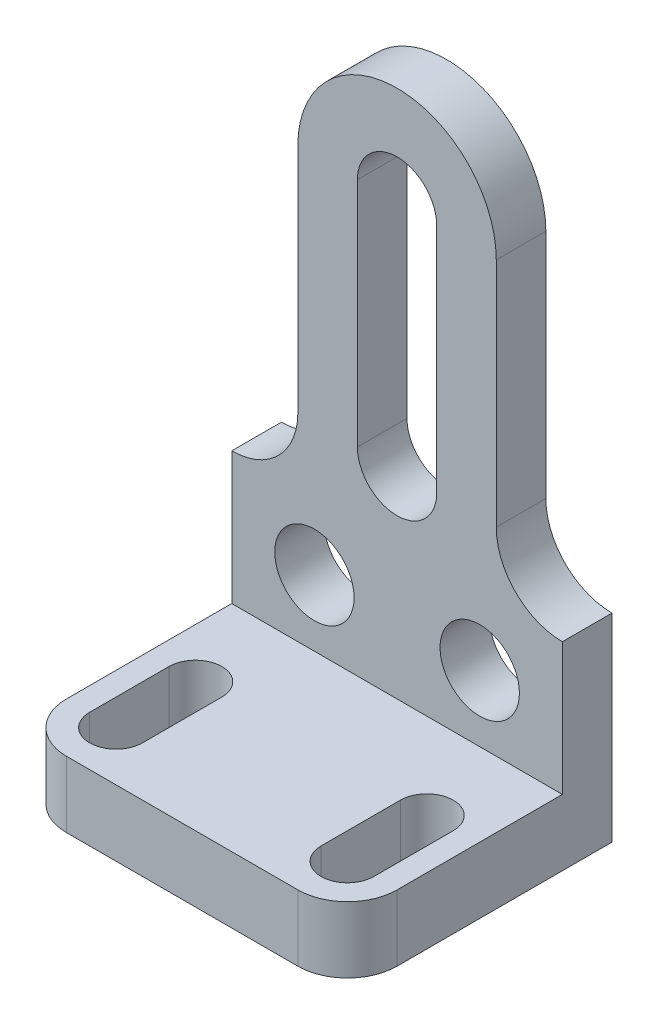
ISO-10303-21;
HEADER;
FILE_DESCRIPTION(('STEP AP214'),'2;1');
FILE_NAME('part.step','',(''),(''),'','','');
FILE_SCHEMA(('AUTOMOTIVE_DESIGN { 1 0 10303 214 1 1 1 1 }'));
ENDSEC;
DATA;
#1=APPLICATION_CONTEXT('core data for automotive mechanical design processes');
#2=APPLICATION_PROTOCOL_DEFINITION('international standard','automotive_design',2000,#1);
#3=PRODUCT_CONTEXT('',#1,'mechanical');
#4=PRODUCT('Part','Part','',(#3));
#5=PRODUCT_RELATED_PRODUCT_CATEGORY('part','',(#4));
#6=PRODUCT_DEFINITION_FORMATION('','',#4);
#7=PRODUCT_DEFINITION_CONTEXT('part definition',#1,'design');
#8=PRODUCT_DEFINITION('design','',#6,#7);
#9=PRODUCT_DEFINITION_SHAPE('','',#8);
#10=(LENGTH_UNIT() NAMED_UNIT(*) SI_UNIT(.MILLI.,.METRE.));
#11=(NAMED_UNIT(*) PLANE_ANGLE_UNIT() SI_UNIT($,.RADIAN.));
#12=(NAMED_UNIT(*) SI_UNIT($,.STERADIAN.) SOLID_ANGLE_UNIT());
#13=UNCERTAINTY_MEASURE_WITH_UNIT(LENGTH_MEASURE(1.E-05),#10,'distance_accuracy_value','');
#14=(GEOMETRIC_REPRESENTATION_CONTEXT(3) GLOBAL_UNCERTAINTY_ASSIGNED_CONTEXT((#13)) GLOBAL_UNIT_ASSIGNED_CONTEXT((#10,
#11,#12)) REPRESENTATION_CONTEXT('',''));
#15=CARTESIAN_POINT('',(0.,0.,0.));
#16=DIRECTION('',(0.,0.,1.));
#17=DIRECTION('',(1.,0.,0.));
#18=AXIS2_PLACEMENT_3D('',#15,#16,#17);
#19=CARTESIAN_POINT('',(0.,150.,15.));
#20=DIRECTION('',(0.,0.,1.));
#21=DIRECTION('',(1.,0.,0.));
#22=AXIS2_PLACEMENT_3D('',#19,#20,#21);
#23=PLANE('',#22);
#24=CARTESIAN_POINT('',(-25.,40.,15.));
#25=DIRECTION('',(0.,0.,1.));
#26=DIRECTION('',(1.,0.,0.));
#27=AXIS2_PLACEMENT_3D('',#24,#25,#26);
#28=CIRCLE('',#27,12.);
#29=CARTESIAN_POINT('',(-13.,40.,15.));
#30=VERTEX_POINT('',#29);
#31=EDGE_CURVE('E318',#30,#30,#28,.T.);
#32=ORIENTED_EDGE('',*,*,#31,.F.);
#33=EDGE_LOOP('',(#32));
#34=FACE_BOUND('',#33,.T.);
#35=DIRECTION('',(0.,-1.,0.));
#36=VECTOR('',#35,1.);
#37=CARTESIAN_POINT('',(-12.,150.,15.));
#38=LINE('',#37,#36);
#39=CARTESIAN_POINT('',(-12.,150.,15.));
#40=VERTEX_POINT('',#39);
#41=CARTESIAN_POINT('',(-12.,80.,15.));
#42=VERTEX_POINT('',#41);
#43=EDGE_CURVE('E326',#40,#42,#38,.T.);
#44=ORIENTED_EDGE('',*,*,#43,.F.);
#45=CARTESIAN_POINT('',(0.,150.,15.));
#46=DIRECTION('',(0.,0.,1.));
#47=DIRECTION('',(1.,0.,0.));
#48=AXIS2_PLACEMENT_3D('',#45,#46,#47);
#49=CIRCLE('',#48,12.);
#50=CARTESIAN_POINT('',(12.,150.,15.));
#51=VERTEX_POINT('',#50);
#52=EDGE_CURVE('E322',#51,#40,#49,.T.);
#53=ORIENTED_EDGE('',*,*,#52,.F.);
#54=DIRECTION('',(0.,1.,0.));
#55=VECTOR('',#54,1.);
#56=CARTESIAN_POINT('',(12.,150.,15.));
#57=LINE('',#56,#55);
#58=CARTESIAN_POINT('',(12.,80.,15.));
#59=VERTEX_POINT('',#58);
#60=EDGE_CURVE('E335',#59,#51,#57,.T.);
#61=ORIENTED_EDGE('',*,*,#60,.F.);
#62=CARTESIAN_POINT('',(0.,80.,15.));
#63=DIRECTION('',(0.,0.,1.));
#64=DIRECTION('',(1.,0.,0.));
#65=AXIS2_PLACEMENT_3D('',#62,#63,#64);
#66=CIRCLE('',#65,12.);
#67=EDGE_CURVE('E328',#42,#59,#66,.T.);
#68=ORIENTED_EDGE('',*,*,#67,.F.);
#69=EDGE_LOOP('',(#44,#53,#61,#68));
#70=FACE_BOUND('',#69,.T.);
#71=CARTESIAN_POINT('',(25.,40.,15.));
#72=DIRECTION('',(0.,0.,1.));
#73=DIRECTION('',(1.,0.,0.));
#74=AXIS2_PLACEMENT_3D('',#71,#72,#73);
#75=CIRCLE('',#74,12.);
#76=CARTESIAN_POINT('',(37.,40.,15.));
#77=VERTEX_POINT('',#76);
#78=EDGE_CURVE('E315',#77,#77,#75,.T.);
#79=ORIENTED_EDGE('',*,*,#78,.F.);
#80=EDGE_LOOP('',(#79));
#81=FACE_BOUND('',#80,.T.);
#82=DIRECTION('',(0.,-1.,0.));
#83=VECTOR('',#82,1.);
#84=CARTESIAN_POINT('',(-50.,0.,15.));
#85=LINE('',#84,#83);
#86=CARTESIAN_POINT('',(-50.,60.,15.));
#87=VERTEX_POINT('',#86);
#88=CARTESIAN_POINT('',(-50.,20.,15.));
#89=VERTEX_POINT('',#88);
#90=EDGE_CURVE('E365',#87,#89,#85,.T.);
#91=ORIENTED_EDGE('',*,*,#90,.T.);
#92=DIRECTION('',(1.,0.,0.));
#93=VECTOR('',#92,1.);
#94=CARTESIAN_POINT('',(50.,20.,15.));
#95=LINE('',#94,#93);
#96=CARTESIAN_POINT('',(50.,20.,15.));
#97=VERTEX_POINT('',#96);
#98=EDGE_CURVE('E295',#89,#97,#95,.T.);
#99=ORIENTED_EDGE('',*,*,#98,.T.);
#100=DIRECTION('',(0.,1.,0.));
#101=VECTOR('',#100,1.);
#102=CARTESIAN_POINT('',(50.,0.,15.));
#103=LINE('',#102,#101);
#104=CARTESIAN_POINT('',(50.,60.,15.));
#105=VERTEX_POINT('',#104);
#106=EDGE_CURVE('E354',#97,#105,#103,.T.);
#107=ORIENTED_EDGE('',*,*,#106,.T.);
#108=CARTESIAN_POINT('',(50.,80.,15.));
#109=DIRECTION('',(0.,0.,1.));
#110=DIRECTION('',(1.,0.,0.));
#111=AXIS2_PLACEMENT_3D('',#108,#109,#110);
#112=CIRCLE('',#111,20.);
#113=CARTESIAN_POINT('',(30.,80.,15.));
#114=VERTEX_POINT('',#113);
#115=EDGE_CURVE('E401',#105,#114,#112,.F.);
#116=ORIENTED_EDGE('',*,*,#115,.T.);
#117=DIRECTION('',(0.,1.,0.));
#118=VECTOR('',#117,1.);
#119=CARTESIAN_POINT('',(30.,150.,15.));
#120=LINE('',#119,#118);
#121=CARTESIAN_POINT('',(30.,150.,15.));
#122=VERTEX_POINT('',#121);
#123=EDGE_CURVE('E360',#114,#122,#120,.T.);
#124=ORIENTED_EDGE('',*,*,#123,.T.);
#125=CARTESIAN_POINT('',(0.,150.,15.));
#126=DIRECTION('',(0.,0.,1.));
#127=DIRECTION('',(1.,0.,0.));
#128=AXIS2_PLACEMENT_3D('',#125,#126,#127);
#129=CIRCLE('',#128,30.);
#130=CARTESIAN_POINT('',(-30.,150.,15.));
#131=VERTEX_POINT('',#130);
#132=EDGE_CURVE('E359',#122,#131,#129,.T.);
#133=ORIENTED_EDGE('',*,*,#132,.T.);
#134=DIRECTION('',(0.,-1.,0.));
#135=VECTOR('',#134,1.);
#136=CARTESIAN_POINT('',(-30.,60.,15.));
#137=LINE('',#136,#135);
#138=CARTESIAN_POINT('',(-30.,80.,15.));
#139=VERTEX_POINT('',#138);
#140=EDGE_CURVE('E362',#131,#139,#137,.T.);
#141=ORIENTED_EDGE('',*,*,#140,.T.);
#142=CARTESIAN_POINT('',(-50.,80.,15.));
#143=DIRECTION('',(0.,0.,1.));
#144=DIRECTION('',(1.,0.,0.));
#145=AXIS2_PLACEMENT_3D('',#142,#143,#144);
#146=CIRCLE('',#145,20.);
#147=EDGE_CURVE('E11',#139,#87,#146,.F.);
#148=ORIENTED_EDGE('',*,*,#147,.T.);
#149=EDGE_LOOP('',(#91,#99,#107,#116,#124,#133,#141,#148));
#150=FACE_BOUND('',#149,.T.);
#151=ADVANCED_FACE('F39',(#34,#70,#81,#150),#23,.T.);
#152=CARTESIAN_POINT('',(0.,150.,0.));
#153=DIRECTION('',(0.,0.,1.));
#154=DIRECTION('',(1.,0.,0.));
#155=AXIS2_PLACEMENT_3D('',#152,#153,#154);
#156=PLANE('',#155);
#157=DIRECTION('',(1.,0.,0.));
#158=VECTOR('',#157,1.);
#159=CARTESIAN_POINT('',(0.,0.,0.));
#160=LINE('',#159,#158);
#161=CARTESIAN_POINT('',(-50.,0.,0.));
#162=VERTEX_POINT('',#161);
#163=CARTESIAN_POINT('',(50.,0.,0.));
#164=VERTEX_POINT('',#163);
#165=EDGE_CURVE('E353',#162,#164,#160,.T.);
#166=ORIENTED_EDGE('',*,*,#165,.F.);
#167=DIRECTION('',(0.,-1.,0.));
#168=VECTOR('',#167,1.);
#169=CARTESIAN_POINT('',(-50.,0.,0.));
#170=LINE('',#169,#168);
#171=CARTESIAN_POINT('',(-50.,60.,0.));
#172=VERTEX_POINT('',#171);
#173=EDGE_CURVE('E357',#172,#162,#170,.T.);
#174=ORIENTED_EDGE('',*,*,#173,.F.);
#175=CARTESIAN_POINT('',(-50.,80.,0.));
#176=DIRECTION('',(0.,0.,1.));
#177=DIRECTION('',(1.,0.,0.));
#178=AXIS2_PLACEMENT_3D('',#175,#176,#177);
#179=CIRCLE('',#178,20.);
#180=CARTESIAN_POINT('',(-30.,80.,0.));
#181=VERTEX_POINT('',#180);
#182=EDGE_CURVE('E50',#172,#181,#179,.T.);
#183=ORIENTED_EDGE('',*,*,#182,.T.);
#184=DIRECTION('',(0.,-1.,0.));
#185=VECTOR('',#184,1.);
#186=CARTESIAN_POINT('',(-30.,60.,0.));
#187=LINE('',#186,#185);
#188=CARTESIAN_POINT('',(-30.,150.,0.));
#189=VERTEX_POINT('',#188);
#190=EDGE_CURVE('E376',#189,#181,#187,.T.);
#191=ORIENTED_EDGE('',*,*,#190,.F.);
#192=CARTESIAN_POINT('',(0.,150.,0.));
#193=DIRECTION('',(0.,0.,1.));
#194=DIRECTION('',(1.,0.,0.));
#195=AXIS2_PLACEMENT_3D('',#192,#193,#194);
#196=CIRCLE('',#195,30.);
#197=CARTESIAN_POINT('',(30.,150.,0.));
#198=VERTEX_POINT('',#197);
#199=EDGE_CURVE('E372',#198,#189,#196,.T.);
#200=ORIENTED_EDGE('',*,*,#199,.F.);
#201=DIRECTION('',(0.,1.,0.));
#202=VECTOR('',#201,1.);
#203=CARTESIAN_POINT('',(30.,150.,0.));
#204=LINE('',#203,#202);
#205=CARTESIAN_POINT('',(30.,80.,0.));
#206=VERTEX_POINT('',#205);
#207=EDGE_CURVE('E375',#206,#198,#204,.T.);
#208=ORIENTED_EDGE('',*,*,#207,.F.);
#209=CARTESIAN_POINT('',(50.,80.,0.));
#210=DIRECTION('',(0.,0.,1.));
#211=DIRECTION('',(1.,0.,0.));
#212=AXIS2_PLACEMENT_3D('',#209,#210,#211);
#213=CIRCLE('',#212,20.);
#214=CARTESIAN_POINT('',(50.,60.,0.));
#215=VERTEX_POINT('',#214);
#216=EDGE_CURVE('E402',#206,#215,#213,.T.);
#217=ORIENTED_EDGE('',*,*,#216,.T.);
#218=DIRECTION('',(0.,1.,0.));
#219=VECTOR('',#218,1.);
#220=CARTESIAN_POINT('',(50.,0.,0.));
#221=LINE('',#220,#219);
#222=EDGE_CURVE('E369',#164,#215,#221,.T.);
#223=ORIENTED_EDGE('',*,*,#222,.F.);
#224=EDGE_LOOP('',(#166,#174,#183,#191,#200,#208,#217,#223));
#225=FACE_BOUND('',#224,.T.);
#226=CARTESIAN_POINT('',(0.,150.,0.));
#227=DIRECTION('',(0.,0.,1.));
#228=DIRECTION('',(1.,0.,0.));
#229=AXIS2_PLACEMENT_3D('',#226,#227,#228);
#230=CIRCLE('',#229,12.);
#231=CARTESIAN_POINT('',(12.,150.,0.));
#232=VERTEX_POINT('',#231);
#233=CARTESIAN_POINT('',(-12.,150.,0.));
#234=VERTEX_POINT('',#233);
#235=EDGE_CURVE('E321',#232,#234,#230,.T.);
#236=ORIENTED_EDGE('',*,*,#235,.T.);
#237=DIRECTION('',(0.,-1.,0.));
#238=VECTOR('',#237,1.);
#239=CARTESIAN_POINT('',(-12.,150.,0.));
#240=LINE('',#239,#238);
#241=CARTESIAN_POINT('',(-12.,80.,0.));
#242=VERTEX_POINT('',#241);
#243=EDGE_CURVE('E340',#234,#242,#240,.T.);
#244=ORIENTED_EDGE('',*,*,#243,.T.);
#245=CARTESIAN_POINT('',(0.,80.,0.));
#246=DIRECTION('',(0.,0.,1.));
#247=DIRECTION('',(1.,0.,0.));
#248=AXIS2_PLACEMENT_3D('',#245,#246,#247);
#249=CIRCLE('',#248,12.);
#250=CARTESIAN_POINT('',(12.,80.,0.));
#251=VERTEX_POINT('',#250);
#252=EDGE_CURVE('E339',#242,#251,#249,.T.);
#253=ORIENTED_EDGE('',*,*,#252,.T.);
#254=DIRECTION('',(0.,1.,0.));
#255=VECTOR('',#254,1.);
#256=CARTESIAN_POINT('',(12.,150.,0.));
#257=LINE('',#256,#255);
#258=EDGE_CURVE('E330',#251,#232,#257,.T.);
#259=ORIENTED_EDGE('',*,*,#258,.T.);
#260=EDGE_LOOP('',(#236,#244,#253,#259));
#261=FACE_BOUND('',#260,.T.);
#262=CARTESIAN_POINT('',(-25.,40.,0.));
#263=DIRECTION('',(0.,0.,1.));
#264=DIRECTION('',(1.,0.,0.));
#265=AXIS2_PLACEMENT_3D('',#262,#263,#264);
#266=CIRCLE('',#265,12.);
#267=CARTESIAN_POINT('',(-13.,40.,0.));
#268=VERTEX_POINT('',#267);
#269=EDGE_CURVE('E312',#268,#268,#266,.T.);
#270=ORIENTED_EDGE('',*,*,#269,.T.);
#271=EDGE_LOOP('',(#270));
#272=FACE_BOUND('',#271,.T.);
#273=CARTESIAN_POINT('',(25.,40.,0.));
#274=DIRECTION('',(0.,0.,1.));
#275=DIRECTION('',(1.,0.,0.));
#276=AXIS2_PLACEMENT_3D('',#273,#274,#275);
#277=CIRCLE('',#276,12.);
#278=CARTESIAN_POINT('',(37.,40.,0.));
#279=VERTEX_POINT('',#278);
#280=EDGE_CURVE('E304',#279,#279,#277,.T.);
#281=ORIENTED_EDGE('',*,*,#280,.T.);
#282=EDGE_LOOP('',(#281));
#283=FACE_BOUND('',#282,.T.);
#284=ADVANCED_FACE('F410',(#225,#261,#272,#283),#156,.F.);
#285=CARTESIAN_POINT('',(0.,0.,15.));
#286=DIRECTION('',(0.,1.,0.));
#287=DIRECTION('',(0.,0.,1.));
#288=AXIS2_PLACEMENT_3D('',#285,#286,#287);
#289=PLANE('',#288);
#290=ORIENTED_EDGE('',*,*,#165,.T.);
#291=DIRECTION('',(0.,0.,-1.));
#292=VECTOR('',#291,1.);
#293=CARTESIAN_POINT('',(50.,0.,15.));
#294=LINE('',#293,#292);
#295=CARTESIAN_POINT('',(50.,0.,65.));
#296=VERTEX_POINT('',#295);
#297=EDGE_CURVE('E393',#296,#164,#294,.T.);
#298=ORIENTED_EDGE('',*,*,#297,.F.);
#299=CARTESIAN_POINT('',(35.,0.,65.));
#300=DIRECTION('',(0.,-1.,0.));
#301=DIRECTION('',(0.,0.,-1.));
#302=AXIS2_PLACEMENT_3D('',#299,#300,#301);
#303=CIRCLE('',#302,15.);
#304=CARTESIAN_POINT('',(35.,0.,80.));
#305=VERTEX_POINT('',#304);
#306=EDGE_CURVE('E275',#296,#305,#303,.T.);
#307=ORIENTED_EDGE('',*,*,#306,.T.);
#308=DIRECTION('',(-1.,0.,0.));
#309=VECTOR('',#308,1.);
#310=CARTESIAN_POINT('',(35.,0.,80.));
#311=LINE('',#310,#309);
#312=CARTESIAN_POINT('',(-35.,0.,80.));
#313=VERTEX_POINT('',#312);
#314=EDGE_CURVE('E300',#305,#313,#311,.T.);
#315=ORIENTED_EDGE('',*,*,#314,.T.);
#316=CARTESIAN_POINT('',(-35.,0.,65.));
#317=DIRECTION('',(0.,-1.,0.));
#318=DIRECTION('',(0.,0.,-1.));
#319=AXIS2_PLACEMENT_3D('',#316,#317,#318);
#320=CIRCLE('',#319,15.);
#321=CARTESIAN_POINT('',(-50.,0.,65.));
#322=VERTEX_POINT('',#321);
#323=EDGE_CURVE('E281',#313,#322,#320,.T.);
#324=ORIENTED_EDGE('',*,*,#323,.T.);
#325=DIRECTION('',(0.,0.,-1.));
#326=VECTOR('',#325,1.);
#327=CARTESIAN_POINT('',(-50.,0.,15.));
#328=LINE('',#327,#326);
#329=EDGE_CURVE('E370',#322,#162,#328,.T.);
#330=ORIENTED_EDGE('',*,*,#329,.T.);
#331=EDGE_LOOP('',(#290,#298,#307,#315,#324,#330));
#332=FACE_BOUND('',#331,.T.);
#333=CARTESIAN_POINT('',(-35.,0.,65.));
#334=DIRECTION('',(0.,-1.,0.));
#335=DIRECTION('',(0.,0.,-1.));
#336=AXIS2_PLACEMENT_3D('',#333,#334,#335);
#337=CIRCLE('',#336,8.00000000000001);
#338=CARTESIAN_POINT('',(-27.,0.,65.));
#339=VERTEX_POINT('',#338);
#340=CARTESIAN_POINT('',(-43.,0.,65.));
#341=VERTEX_POINT('',#340);
#342=EDGE_CURVE('E209',#339,#341,#337,.T.);
#343=ORIENTED_EDGE('',*,*,#342,.F.);
#344=DIRECTION('',(0.,0.,1.));
#345=VECTOR('',#344,1.);
#346=CARTESIAN_POINT('',(-27.,0.,65.));
#347=LINE('',#346,#345);
#348=CARTESIAN_POINT('',(-27.,0.,41.));
#349=VERTEX_POINT('',#348);
#350=EDGE_CURVE('E227',#349,#339,#347,.T.);
#351=ORIENTED_EDGE('',*,*,#350,.F.);
#352=CARTESIAN_POINT('',(-35.,0.,41.));
#353=DIRECTION('',(0.,-1.,0.));
#354=DIRECTION('',(0.,0.,-1.));
#355=AXIS2_PLACEMENT_3D('',#352,#353,#354);
#356=CIRCLE('',#355,8.00000000000001);
#357=CARTESIAN_POINT('',(-43.,0.,41.));
#358=VERTEX_POINT('',#357);
#359=EDGE_CURVE('E231',#358,#349,#356,.T.);
#360=ORIENTED_EDGE('',*,*,#359,.F.);
#361=DIRECTION('',(0.,0.,-1.));
#362=VECTOR('',#361,1.);
#363=CARTESIAN_POINT('',(-43.,0.,65.));
#364=LINE('',#363,#362);
#365=EDGE_CURVE('E240',#341,#358,#364,.T.);
#366=ORIENTED_EDGE('',*,*,#365,.F.);
#367=EDGE_LOOP('',(#343,#351,#360,#366));
#368=FACE_BOUND('',#367,.T.);
#369=CARTESIAN_POINT('',(35.,0.,65.));
#370=DIRECTION('',(0.,-1.,0.));
#371=DIRECTION('',(0.,0.,-1.));
#372=AXIS2_PLACEMENT_3D('',#369,#370,#371);
#373=CIRCLE('',#372,8.00000000000001);
#374=CARTESIAN_POINT('',(43.,0.,65.));
#375=VERTEX_POINT('',#374);
#376=CARTESIAN_POINT('',(27.,0.,65.));
#377=VERTEX_POINT('',#376);
#378=EDGE_CURVE('E242',#375,#377,#373,.T.);
#379=ORIENTED_EDGE('',*,*,#378,.F.);
#380=DIRECTION('',(0.,0.,1.));
#381=VECTOR('',#380,1.);
#382=CARTESIAN_POINT('',(43.,0.,65.));
#383=LINE('',#382,#381);
#384=CARTESIAN_POINT('',(43.,0.,41.));
#385=VERTEX_POINT('',#384);
#386=EDGE_CURVE('E253',#385,#375,#383,.T.);
#387=ORIENTED_EDGE('',*,*,#386,.F.);
#388=CARTESIAN_POINT('',(35.,0.,41.));
#389=DIRECTION('',(0.,-1.,0.));
#390=DIRECTION('',(0.,0.,-1.));
#391=AXIS2_PLACEMENT_3D('',#388,#389,#390);
#392=CIRCLE('',#391,8.);
#393=CARTESIAN_POINT('',(27.,0.,41.));
#394=VERTEX_POINT('',#393);
#395=EDGE_CURVE('E264',#394,#385,#392,.T.);
#396=ORIENTED_EDGE('',*,*,#395,.F.);
#397=DIRECTION('',(0.,0.,-1.));
#398=VECTOR('',#397,1.);
#399=CARTESIAN_POINT('',(27.,0.,65.));
#400=LINE('',#399,#398);
#401=EDGE_CURVE('E265',#377,#394,#400,.T.);
#402=ORIENTED_EDGE('',*,*,#401,.F.);
#403=EDGE_LOOP('',(#379,#387,#396,#402));
#404=FACE_BOUND('',#403,.T.);
#405=ADVANCED_FACE('F438',(#332,#368,#404),#289,.F.);
#406=CARTESIAN_POINT('',(50.,0.,15.));
#407=DIRECTION('',(-1.,0.,0.));
#408=DIRECTION('',(0.,0.,1.));
#409=AXIS2_PLACEMENT_3D('',#406,#407,#408);
#410=PLANE('',#409);
#411=ORIENTED_EDGE('',*,*,#222,.T.);
#412=DIRECTION('',(0.,0.,-1.));
#413=VECTOR('',#412,1.);
#414=CARTESIAN_POINT('',(50.,60.,15.));
#415=LINE('',#414,#413);
#416=EDGE_CURVE('E391',#105,#215,#415,.T.);
#417=ORIENTED_EDGE('',*,*,#416,.F.);
#418=ORIENTED_EDGE('',*,*,#106,.F.);
#419=DIRECTION('',(0.,0.,1.));
#420=VECTOR('',#419,1.);
#421=CARTESIAN_POINT('',(50.,20.,15.));
#422=LINE('',#421,#420);
#423=CARTESIAN_POINT('',(50.,20.,65.));
#424=VERTEX_POINT('',#423);
#425=EDGE_CURVE('E53',#97,#424,#422,.T.);
#426=ORIENTED_EDGE('',*,*,#425,.T.);
#427=DIRECTION('',(0.,-1.,0.));
#428=VECTOR('',#427,1.);
#429=CARTESIAN_POINT('',(50.,20.,65.));
#430=LINE('',#429,#428);
#431=EDGE_CURVE('E294',#424,#296,#430,.T.);
#432=ORIENTED_EDGE('',*,*,#431,.T.);
#433=ORIENTED_EDGE('',*,*,#297,.T.);
#434=EDGE_LOOP('',(#411,#417,#418,#426,#432,#433));
#435=FACE_BOUND('',#434,.T.);
#436=ADVANCED_FACE('F424',(#435),#410,.F.);
#437=CARTESIAN_POINT('',(30.,150.,15.));
#438=DIRECTION('',(-1.,0.,0.));
#439=DIRECTION('',(0.,-1.,0.));
#440=AXIS2_PLACEMENT_3D('',#437,#438,#439);
#441=PLANE('',#440);
#442=ORIENTED_EDGE('',*,*,#123,.F.);
#443=DIRECTION('',(0.,0.,-1.));
#444=VECTOR('',#443,1.);
#445=CARTESIAN_POINT('',(30.,80.,0.));
#446=LINE('',#445,#444);
#447=EDGE_CURVE('E400',#114,#206,#446,.T.);
#448=ORIENTED_EDGE('',*,*,#447,.T.);
#449=ORIENTED_EDGE('',*,*,#207,.T.);
#450=DIRECTION('',(0.,0.,-1.));
#451=VECTOR('',#450,1.);
#452=CARTESIAN_POINT('',(30.,150.,15.));
#453=LINE('',#452,#451);
#454=EDGE_CURVE('E389',#122,#198,#453,.T.);
#455=ORIENTED_EDGE('',*,*,#454,.F.);
#456=EDGE_LOOP('',(#442,#448,#449,#455));
#457=FACE_BOUND('',#456,.T.);
#458=ADVANCED_FACE('F433',(#457),#441,.F.);
#459=CARTESIAN_POINT('',(0.,150.,15.));
#460=DIRECTION('',(0.,0.,-1.));
#461=DIRECTION('',(-1.,0.,0.));
#462=AXIS2_PLACEMENT_3D('',#459,#460,#461);
#463=CYLINDRICAL_SURFACE('',#462,30.);
#464=ORIENTED_EDGE('',*,*,#199,.T.);
#465=DIRECTION('',(0.,0.,-1.));
#466=VECTOR('',#465,1.);
#467=CARTESIAN_POINT('',(-30.,150.,15.));
#468=LINE('',#467,#466);
#469=EDGE_CURVE('E384',#131,#189,#468,.T.);
#470=ORIENTED_EDGE('',*,*,#469,.F.);
#471=ORIENTED_EDGE('',*,*,#132,.F.);
#472=ORIENTED_EDGE('',*,*,#454,.T.);
#473=EDGE_LOOP('',(#464,#470,#471,#472));
#474=FACE_BOUND('',#473,.T.);
#475=ADVANCED_FACE('F440',(#474),#463,.T.);
#476=CARTESIAN_POINT('',(-30.,60.,15.));
#477=DIRECTION('',(1.,0.,0.));
#478=DIRECTION('',(0.,0.,-1.));
#479=AXIS2_PLACEMENT_3D('',#476,#477,#478);
#480=PLANE('',#479);
#481=ORIENTED_EDGE('',*,*,#190,.T.);
#482=DIRECTION('',(0.,0.,-1.));
#483=VECTOR('',#482,1.);
#484=CARTESIAN_POINT('',(-30.,80.,15.));
#485=LINE('',#484,#483);
#486=EDGE_CURVE('E65',#181,#139,#485,.F.);
#487=ORIENTED_EDGE('',*,*,#486,.T.);
#488=ORIENTED_EDGE('',*,*,#140,.F.);
#489=ORIENTED_EDGE('',*,*,#469,.T.);
#490=EDGE_LOOP('',(#481,#487,#488,#489));
#491=FACE_BOUND('',#490,.T.);
#492=ADVANCED_FACE('F415',(#491),#480,.F.);
#493=CARTESIAN_POINT('',(-50.,0.,15.));
#494=DIRECTION('',(1.,0.,0.));
#495=DIRECTION('',(0.,0.,-1.));
#496=AXIS2_PLACEMENT_3D('',#493,#494,#495);
#497=PLANE('',#496);
#498=ORIENTED_EDGE('',*,*,#173,.T.);
#499=ORIENTED_EDGE('',*,*,#329,.F.);
#500=DIRECTION('',(0.,-1.,0.));
#501=VECTOR('',#500,1.);
#502=CARTESIAN_POINT('',(-50.,20.,65.));
#503=LINE('',#502,#501);
#504=CARTESIAN_POINT('',(-50.,20.,65.));
#505=VERTEX_POINT('',#504);
#506=EDGE_CURVE('E305',#505,#322,#503,.T.);
#507=ORIENTED_EDGE('',*,*,#506,.F.);
#508=DIRECTION('',(0.,0.,-1.));
#509=VECTOR('',#508,1.);
#510=CARTESIAN_POINT('',(-50.,20.,15.));
#511=LINE('',#510,#509);
#512=EDGE_CURVE('E289',#505,#89,#511,.T.);
#513=ORIENTED_EDGE('',*,*,#512,.T.);
#514=ORIENTED_EDGE('',*,*,#90,.F.);
#515=DIRECTION('',(0.,0.,-1.));
#516=VECTOR('',#515,1.);
#517=CARTESIAN_POINT('',(-50.,60.,15.));
#518=LINE('',#517,#516);
#519=EDGE_CURVE('E385',#87,#172,#518,.T.);
#520=ORIENTED_EDGE('',*,*,#519,.T.);
#521=EDGE_LOOP('',(#498,#499,#507,#513,#514,#520));
#522=FACE_BOUND('',#521,.T.);
#523=ADVANCED_FACE('F416',(#522),#497,.F.);
#524=CARTESIAN_POINT('',(0.,150.,15.));
#525=DIRECTION('',(0.,0.,-1.));
#526=DIRECTION('',(-1.,0.,0.));
#527=AXIS2_PLACEMENT_3D('',#524,#525,#526);
#528=CYLINDRICAL_SURFACE('',#527,12.);
#529=ORIENTED_EDGE('',*,*,#235,.F.);
#530=DIRECTION('',(0.,0.,-1.));
#531=VECTOR('',#530,1.);
#532=CARTESIAN_POINT('',(12.,150.,15.));
#533=LINE('',#532,#531);
#534=EDGE_CURVE('E331',#51,#232,#533,.T.);
#535=ORIENTED_EDGE('',*,*,#534,.F.);
#536=ORIENTED_EDGE('',*,*,#52,.T.);
#537=DIRECTION('',(0.,0.,-1.));
#538=VECTOR('',#537,1.);
#539=CARTESIAN_POINT('',(-12.,150.,15.));
#540=LINE('',#539,#538);
#541=EDGE_CURVE('E351',#40,#234,#540,.T.);
#542=ORIENTED_EDGE('',*,*,#541,.T.);
#543=EDGE_LOOP('',(#529,#535,#536,#542));
#544=FACE_BOUND('',#543,.T.);
#545=ADVANCED_FACE('F471',(#544),#528,.F.);
#546=CARTESIAN_POINT('',(-12.,150.,15.));
#547=DIRECTION('',(1.,0.,0.));
#548=DIRECTION('',(0.,1.,0.));
#549=AXIS2_PLACEMENT_3D('',#546,#547,#548);
#550=PLANE('',#549);
#551=ORIENTED_EDGE('',*,*,#243,.F.);
#552=ORIENTED_EDGE('',*,*,#541,.F.);
#553=ORIENTED_EDGE('',*,*,#43,.T.);
#554=DIRECTION('',(0.,0.,-1.));
#555=VECTOR('',#554,1.);
#556=CARTESIAN_POINT('',(-12.,80.,15.));
#557=LINE('',#556,#555);
#558=EDGE_CURVE('E349',#42,#242,#557,.T.);
#559=ORIENTED_EDGE('',*,*,#558,.T.);
#560=EDGE_LOOP('',(#551,#552,#553,#559));
#561=FACE_BOUND('',#560,.T.);
#562=ADVANCED_FACE('F506',(#561),#550,.T.);
#563=CARTESIAN_POINT('',(0.,80.,15.));
#564=DIRECTION('',(0.,0.,-1.));
#565=DIRECTION('',(-1.,0.,0.));
#566=AXIS2_PLACEMENT_3D('',#563,#564,#565);
#567=CYLINDRICAL_SURFACE('',#566,12.);
#568=ORIENTED_EDGE('',*,*,#252,.F.);
#569=ORIENTED_EDGE('',*,*,#558,.F.);
#570=ORIENTED_EDGE('',*,*,#67,.T.);
#571=DIRECTION('',(0.,0.,-1.));
#572=VECTOR('',#571,1.);
#573=CARTESIAN_POINT('',(12.,80.,15.));
#574=LINE('',#573,#572);
#575=EDGE_CURVE('E350',#59,#251,#574,.T.);
#576=ORIENTED_EDGE('',*,*,#575,.T.);
#577=EDGE_LOOP('',(#568,#569,#570,#576));
#578=FACE_BOUND('',#577,.T.);
#579=ADVANCED_FACE('F502',(#578),#567,.F.);
#580=CARTESIAN_POINT('',(12.,150.,15.));
#581=DIRECTION('',(-1.,0.,0.));
#582=DIRECTION('',(0.,-1.,0.));
#583=AXIS2_PLACEMENT_3D('',#580,#581,#582);
#584=PLANE('',#583);
#585=ORIENTED_EDGE('',*,*,#258,.F.);
#586=ORIENTED_EDGE('',*,*,#575,.F.);
#587=ORIENTED_EDGE('',*,*,#60,.T.);
#588=ORIENTED_EDGE('',*,*,#534,.T.);
#589=EDGE_LOOP('',(#585,#586,#587,#588));
#590=FACE_BOUND('',#589,.T.);
#591=ADVANCED_FACE('F497',(#590),#584,.T.);
#592=CARTESIAN_POINT('',(-25.,40.,15.));
#593=DIRECTION('',(0.,0.,-1.));
#594=DIRECTION('',(-1.,0.,0.));
#595=AXIS2_PLACEMENT_3D('',#592,#593,#594);
#596=CYLINDRICAL_SURFACE('',#595,12.);
#597=ORIENTED_EDGE('',*,*,#31,.T.);
#598=EDGE_LOOP('',(#597));
#599=FACE_BOUND('',#598,.T.);
#600=ORIENTED_EDGE('',*,*,#269,.F.);
#601=EDGE_LOOP('',(#600));
#602=FACE_BOUND('',#601,.T.);
#603=ADVANCED_FACE('F491',(#599,#602),#596,.F.);
#604=CARTESIAN_POINT('',(25.,40.,15.));
#605=DIRECTION('',(0.,0.,-1.));
#606=DIRECTION('',(-1.,0.,0.));
#607=AXIS2_PLACEMENT_3D('',#604,#605,#606);
#608=CYLINDRICAL_SURFACE('',#607,12.);
#609=ORIENTED_EDGE('',*,*,#78,.T.);
#610=EDGE_LOOP('',(#609));
#611=FACE_BOUND('',#610,.T.);
#612=ORIENTED_EDGE('',*,*,#280,.F.);
#613=EDGE_LOOP('',(#612));
#614=FACE_BOUND('',#613,.T.);
#615=ADVANCED_FACE('F490',(#611,#614),#608,.F.);
#616=CARTESIAN_POINT('',(50.,80.,15.));
#617=DIRECTION('',(0.,0.,1.));
#618=DIRECTION('',(1.,0.,0.));
#619=AXIS2_PLACEMENT_3D('',#616,#617,#618);
#620=CYLINDRICAL_SURFACE('',#619,20.);
#621=ORIENTED_EDGE('',*,*,#115,.F.);
#622=ORIENTED_EDGE('',*,*,#416,.T.);
#623=ORIENTED_EDGE('',*,*,#216,.F.);
#624=ORIENTED_EDGE('',*,*,#447,.F.);
#625=EDGE_LOOP('',(#621,#622,#623,#624));
#626=FACE_BOUND('',#625,.T.);
#627=ADVANCED_FACE('F427',(#626),#620,.F.);
#628=CARTESIAN_POINT('',(-50.,80.,15.));
#629=DIRECTION('',(0.,0.,1.));
#630=DIRECTION('',(1.,0.,0.));
#631=AXIS2_PLACEMENT_3D('',#628,#629,#630);
#632=CYLINDRICAL_SURFACE('',#631,20.);
#633=ORIENTED_EDGE('',*,*,#147,.F.);
#634=ORIENTED_EDGE('',*,*,#486,.F.);
#635=ORIENTED_EDGE('',*,*,#182,.F.);
#636=ORIENTED_EDGE('',*,*,#519,.F.);
#637=EDGE_LOOP('',(#633,#634,#635,#636));
#638=FACE_BOUND('',#637,.T.);
#639=ADVANCED_FACE('F41',(#638),#632,.F.);
#640=CARTESIAN_POINT('',(-35.,20.,65.));
#641=DIRECTION('',(0.,-1.,0.));
#642=DIRECTION('',(0.,0.,-1.));
#643=AXIS2_PLACEMENT_3D('',#640,#641,#642);
#644=CYLINDRICAL_SURFACE('',#643,15.);
#645=ORIENTED_EDGE('',*,*,#323,.F.);
#646=DIRECTION('',(0.,-1.,0.));
#647=VECTOR('',#646,1.);
#648=CARTESIAN_POINT('',(-35.,20.,80.));
#649=LINE('',#648,#647);
#650=CARTESIAN_POINT('',(-35.,20.,80.));
#651=VERTEX_POINT('',#650);
#652=EDGE_CURVE('E308',#651,#313,#649,.T.);
#653=ORIENTED_EDGE('',*,*,#652,.F.);
#654=CARTESIAN_POINT('',(-35.,20.,65.));
#655=DIRECTION('',(0.,-1.,0.));
#656=DIRECTION('',(0.,0.,-1.));
#657=AXIS2_PLACEMENT_3D('',#654,#655,#656);
#658=CIRCLE('',#657,15.);
#659=EDGE_CURVE('E290',#651,#505,#658,.T.);
#660=ORIENTED_EDGE('',*,*,#659,.T.);
#661=ORIENTED_EDGE('',*,*,#506,.T.);
#662=EDGE_LOOP('',(#645,#653,#660,#661));
#663=FACE_BOUND('',#662,.T.);
#664=ADVANCED_FACE('F441',(#663),#644,.T.);
#665=CARTESIAN_POINT('',(35.,20.,80.));
#666=DIRECTION('',(0.,0.,1.));
#667=DIRECTION('',(1.,0.,0.));
#668=AXIS2_PLACEMENT_3D('',#665,#666,#667);
#669=PLANE('',#668);
#670=ORIENTED_EDGE('',*,*,#314,.F.);
#671=DIRECTION('',(0.,-1.,0.));
#672=VECTOR('',#671,1.);
#673=CARTESIAN_POINT('',(35.,20.,80.));
#674=LINE('',#673,#672);
#675=CARTESIAN_POINT('',(35.,20.,80.));
#676=VERTEX_POINT('',#675);
#677=EDGE_CURVE('E306',#676,#305,#674,.T.);
#678=ORIENTED_EDGE('',*,*,#677,.F.);
#679=DIRECTION('',(-1.,0.,0.));
#680=VECTOR('',#679,1.);
#681=CARTESIAN_POINT('',(35.,20.,80.));
#682=LINE('',#681,#680);
#683=EDGE_CURVE('E283',#676,#651,#682,.T.);
#684=ORIENTED_EDGE('',*,*,#683,.T.);
#685=ORIENTED_EDGE('',*,*,#652,.T.);
#686=EDGE_LOOP('',(#670,#678,#684,#685));
#687=FACE_BOUND('',#686,.T.);
#688=ADVANCED_FACE('F450',(#687),#669,.T.);
#689=CARTESIAN_POINT('',(35.,20.,65.));
#690=DIRECTION('',(0.,-1.,0.));
#691=DIRECTION('',(0.,0.,-1.));
#692=AXIS2_PLACEMENT_3D('',#689,#690,#691);
#693=CYLINDRICAL_SURFACE('',#692,15.);
#694=ORIENTED_EDGE('',*,*,#306,.F.);
#695=ORIENTED_EDGE('',*,*,#431,.F.);
#696=CARTESIAN_POINT('',(35.,20.,65.));
#697=DIRECTION('',(0.,-1.,0.));
#698=DIRECTION('',(0.,0.,-1.));
#699=AXIS2_PLACEMENT_3D('',#696,#697,#698);
#700=CIRCLE('',#699,15.);
#701=EDGE_CURVE('E278',#424,#676,#700,.T.);
#702=ORIENTED_EDGE('',*,*,#701,.T.);
#703=ORIENTED_EDGE('',*,*,#677,.T.);
#704=EDGE_LOOP('',(#694,#695,#702,#703));
#705=FACE_BOUND('',#704,.T.);
#706=ADVANCED_FACE('F449',(#705),#693,.T.);
#707=CARTESIAN_POINT('',(35.,20.,65.));
#708=DIRECTION('',(0.,-1.,0.));
#709=DIRECTION('',(0.,0.,-1.));
#710=AXIS2_PLACEMENT_3D('',#707,#708,#709);
#711=PLANE('',#710);
#712=DIRECTION('',(0.,0.,1.));
#713=VECTOR('',#712,1.);
#714=CARTESIAN_POINT('',(-27.,20.,65.));
#715=LINE('',#714,#713);
#716=CARTESIAN_POINT('',(-27.,20.,41.));
#717=VERTEX_POINT('',#716);
#718=CARTESIAN_POINT('',(-27.,20.,65.));
#719=VERTEX_POINT('',#718);
#720=EDGE_CURVE('E214',#717,#719,#715,.T.);
#721=ORIENTED_EDGE('',*,*,#720,.T.);
#722=CARTESIAN_POINT('',(-35.,20.,65.));
#723=DIRECTION('',(0.,-1.,0.));
#724=DIRECTION('',(0.,0.,-1.));
#725=AXIS2_PLACEMENT_3D('',#722,#723,#724);
#726=CIRCLE('',#725,8.00000000000001);
#727=CARTESIAN_POINT('',(-43.,20.,65.));
#728=VERTEX_POINT('',#727);
#729=EDGE_CURVE('E210',#719,#728,#726,.T.);
#730=ORIENTED_EDGE('',*,*,#729,.T.);
#731=DIRECTION('',(0.,0.,-1.));
#732=VECTOR('',#731,1.);
#733=CARTESIAN_POINT('',(-43.,20.,65.));
#734=LINE('',#733,#732);
#735=CARTESIAN_POINT('',(-43.,20.,41.));
#736=VERTEX_POINT('',#735);
#737=EDGE_CURVE('E218',#728,#736,#734,.T.);
#738=ORIENTED_EDGE('',*,*,#737,.T.);
#739=CARTESIAN_POINT('',(-35.,20.,41.));
#740=DIRECTION('',(0.,-1.,0.));
#741=DIRECTION('',(0.,0.,-1.));
#742=AXIS2_PLACEMENT_3D('',#739,#740,#741);
#743=CIRCLE('',#742,8.00000000000001);
#744=EDGE_CURVE('E224',#736,#717,#743,.T.);
#745=ORIENTED_EDGE('',*,*,#744,.T.);
#746=EDGE_LOOP('',(#721,#730,#738,#745));
#747=FACE_BOUND('',#746,.T.);
#748=DIRECTION('',(0.,0.,1.));
#749=VECTOR('',#748,1.);
#750=CARTESIAN_POINT('',(43.,20.,65.));
#751=LINE('',#750,#749);
#752=CARTESIAN_POINT('',(43.,20.,41.));
#753=VERTEX_POINT('',#752);
#754=CARTESIAN_POINT('',(43.,20.,65.));
#755=VERTEX_POINT('',#754);
#756=EDGE_CURVE('E260',#753,#755,#751,.T.);
#757=ORIENTED_EDGE('',*,*,#756,.T.);
#758=CARTESIAN_POINT('',(35.,20.,65.));
#759=DIRECTION('',(0.,-1.,0.));
#760=DIRECTION('',(0.,0.,-1.));
#761=AXIS2_PLACEMENT_3D('',#758,#759,#760);
#762=CIRCLE('',#761,8.00000000000001);
#763=CARTESIAN_POINT('',(27.,20.,65.));
#764=VERTEX_POINT('',#763);
#765=EDGE_CURVE('E250',#755,#764,#762,.T.);
#766=ORIENTED_EDGE('',*,*,#765,.T.);
#767=DIRECTION('',(0.,0.,-1.));
#768=VECTOR('',#767,1.);
#769=CARTESIAN_POINT('',(27.,20.,65.));
#770=LINE('',#769,#768);
#771=CARTESIAN_POINT('',(27.,20.,41.));
#772=VERTEX_POINT('',#771);
#773=EDGE_CURVE('E249',#764,#772,#770,.T.);
#774=ORIENTED_EDGE('',*,*,#773,.T.);
#775=CARTESIAN_POINT('',(35.,20.,41.));
#776=DIRECTION('',(0.,-1.,0.));
#777=DIRECTION('',(0.,0.,-1.));
#778=AXIS2_PLACEMENT_3D('',#775,#776,#777);
#779=CIRCLE('',#778,8.);
#780=EDGE_CURVE('E255',#772,#753,#779,.T.);
#781=ORIENTED_EDGE('',*,*,#780,.T.);
#782=EDGE_LOOP('',(#757,#766,#774,#781));
#783=FACE_BOUND('',#782,.T.);
#784=ORIENTED_EDGE('',*,*,#425,.F.);
#785=ORIENTED_EDGE('',*,*,#98,.F.);
#786=ORIENTED_EDGE('',*,*,#512,.F.);
#787=ORIENTED_EDGE('',*,*,#659,.F.);
#788=ORIENTED_EDGE('',*,*,#683,.F.);
#789=ORIENTED_EDGE('',*,*,#701,.F.);
#790=EDGE_LOOP('',(#784,#785,#786,#787,#788,#789));
#791=FACE_BOUND('',#790,.T.);
#792=ADVANCED_FACE('F223',(#747,#783,#791),#711,.F.);
#793=CARTESIAN_POINT('',(35.,20.,65.));
#794=DIRECTION('',(0.,-1.,0.));
#795=DIRECTION('',(0.,0.,-1.));
#796=AXIS2_PLACEMENT_3D('',#793,#794,#795);
#797=CYLINDRICAL_SURFACE('',#796,8.00000000000001);
#798=ORIENTED_EDGE('',*,*,#378,.T.);
#799=DIRECTION('',(0.,-1.,0.));
#800=VECTOR('',#799,1.);
#801=CARTESIAN_POINT('',(27.,20.,65.));
#802=LINE('',#801,#800);
#803=EDGE_CURVE('E257',#764,#377,#802,.T.);
#804=ORIENTED_EDGE('',*,*,#803,.F.);
#805=ORIENTED_EDGE('',*,*,#765,.F.);
#806=DIRECTION('',(0.,-1.,0.));
#807=VECTOR('',#806,1.);
#808=CARTESIAN_POINT('',(43.,20.,65.));
#809=LINE('',#808,#807);
#810=EDGE_CURVE('E269',#755,#375,#809,.T.);
#811=ORIENTED_EDGE('',*,*,#810,.T.);
#812=EDGE_LOOP('',(#798,#804,#805,#811));
#813=FACE_BOUND('',#812,.T.);
#814=ADVANCED_FACE('F460',(#813),#797,.F.);
#815=CARTESIAN_POINT('',(43.,20.,65.));
#816=DIRECTION('',(1.,0.,0.));
#817=DIRECTION('',(0.,0.,-1.));
#818=AXIS2_PLACEMENT_3D('',#815,#816,#817);
#819=PLANE('',#818);
#820=ORIENTED_EDGE('',*,*,#386,.T.);
#821=ORIENTED_EDGE('',*,*,#810,.F.);
#822=ORIENTED_EDGE('',*,*,#756,.F.);
#823=DIRECTION('',(0.,-1.,0.));
#824=VECTOR('',#823,1.);
#825=CARTESIAN_POINT('',(43.,20.,41.));
#826=LINE('',#825,#824);
#827=EDGE_CURVE('E272',#753,#385,#826,.T.);
#828=ORIENTED_EDGE('',*,*,#827,.T.);
#829=EDGE_LOOP('',(#820,#821,#822,#828));
#830=FACE_BOUND('',#829,.T.);
#831=ADVANCED_FACE('F594',(#830),#819,.F.);
#832=CARTESIAN_POINT('',(35.,20.,41.));
#833=DIRECTION('',(0.,-1.,0.));
#834=DIRECTION('',(0.,0.,-1.));
#835=AXIS2_PLACEMENT_3D('',#832,#833,#834);
#836=CYLINDRICAL_SURFACE('',#835,8.);
#837=ORIENTED_EDGE('',*,*,#395,.T.);
#838=ORIENTED_EDGE('',*,*,#827,.F.);
#839=ORIENTED_EDGE('',*,*,#780,.F.);
#840=DIRECTION('',(0.,-1.,0.));
#841=VECTOR('',#840,1.);
#842=CARTESIAN_POINT('',(27.,20.,41.));
#843=LINE('',#842,#841);
#844=EDGE_CURVE('E274',#772,#394,#843,.T.);
#845=ORIENTED_EDGE('',*,*,#844,.T.);
#846=EDGE_LOOP('',(#837,#838,#839,#845));
#847=FACE_BOUND('',#846,.T.);
#848=ADVANCED_FACE('F604',(#847),#836,.F.);
#849=CARTESIAN_POINT('',(27.,20.,65.));
#850=DIRECTION('',(-1.,0.,0.));
#851=DIRECTION('',(0.,0.,1.));
#852=AXIS2_PLACEMENT_3D('',#849,#850,#851);
#853=PLANE('',#852);
#854=ORIENTED_EDGE('',*,*,#401,.T.);
#855=ORIENTED_EDGE('',*,*,#844,.F.);
#856=ORIENTED_EDGE('',*,*,#773,.F.);
#857=ORIENTED_EDGE('',*,*,#803,.T.);
#858=EDGE_LOOP('',(#854,#855,#856,#857));
#859=FACE_BOUND('',#858,.T.);
#860=ADVANCED_FACE('F614',(#859),#853,.F.);
#861=CARTESIAN_POINT('',(-35.,20.,65.));
#862=DIRECTION('',(0.,-1.,0.));
#863=DIRECTION('',(0.,0.,-1.));
#864=AXIS2_PLACEMENT_3D('',#861,#862,#863);
#865=CYLINDRICAL_SURFACE('',#864,8.00000000000001);
#866=ORIENTED_EDGE('',*,*,#342,.T.);
#867=DIRECTION('',(0.,-1.,0.));
#868=VECTOR('',#867,1.);
#869=CARTESIAN_POINT('',(-43.,20.,65.));
#870=LINE('',#869,#868);
#871=EDGE_CURVE('E201',#728,#341,#870,.T.);
#872=ORIENTED_EDGE('',*,*,#871,.F.);
#873=ORIENTED_EDGE('',*,*,#729,.F.);
#874=DIRECTION('',(0.,-1.,0.));
#875=VECTOR('',#874,1.);
#876=CARTESIAN_POINT('',(-27.,20.,65.));
#877=LINE('',#876,#875);
#878=EDGE_CURVE('E241',#719,#339,#877,.T.);
#879=ORIENTED_EDGE('',*,*,#878,.T.);
#880=EDGE_LOOP('',(#866,#872,#873,#879));
#881=FACE_BOUND('',#880,.T.);
#882=ADVANCED_FACE('F202',(#881),#865,.F.);
#883=CARTESIAN_POINT('',(-27.,20.,65.));
#884=DIRECTION('',(1.,0.,0.));
#885=DIRECTION('',(0.,0.,-1.));
#886=AXIS2_PLACEMENT_3D('',#883,#884,#885);
#887=PLANE('',#886);
#888=ORIENTED_EDGE('',*,*,#350,.T.);
#889=ORIENTED_EDGE('',*,*,#878,.F.);
#890=ORIENTED_EDGE('',*,*,#720,.F.);
#891=DIRECTION('',(0.,-1.,0.));
#892=VECTOR('',#891,1.);
#893=CARTESIAN_POINT('',(-27.,20.,41.));
#894=LINE('',#893,#892);
#895=EDGE_CURVE('E243',#717,#349,#894,.T.);
#896=ORIENTED_EDGE('',*,*,#895,.T.);
#897=EDGE_LOOP('',(#888,#889,#890,#896));
#898=FACE_BOUND('',#897,.T.);
#899=ADVANCED_FACE('F633',(#898),#887,.F.);
#900=CARTESIAN_POINT('',(-35.,20.,41.));
#901=DIRECTION('',(0.,-1.,0.));
#902=DIRECTION('',(0.,0.,-1.));
#903=AXIS2_PLACEMENT_3D('',#900,#901,#902);
#904=CYLINDRICAL_SURFACE('',#903,8.00000000000001);
#905=ORIENTED_EDGE('',*,*,#359,.T.);
#906=ORIENTED_EDGE('',*,*,#895,.F.);
#907=ORIENTED_EDGE('',*,*,#744,.F.);
#908=DIRECTION('',(0.,-1.,0.));
#909=VECTOR('',#908,1.);
#910=CARTESIAN_POINT('',(-43.,20.,41.));
#911=LINE('',#910,#909);
#912=EDGE_CURVE('E212',#736,#358,#911,.T.);
#913=ORIENTED_EDGE('',*,*,#912,.T.);
#914=EDGE_LOOP('',(#905,#906,#907,#913));
#915=FACE_BOUND('',#914,.T.);
#916=ADVANCED_FACE('F641',(#915),#904,.F.);
#917=CARTESIAN_POINT('',(-43.,20.,65.));
#918=DIRECTION('',(-1.,0.,0.));
#919=DIRECTION('',(0.,0.,1.));
#920=AXIS2_PLACEMENT_3D('',#917,#918,#919);
#921=PLANE('',#920);
#922=ORIENTED_EDGE('',*,*,#365,.T.);
#923=ORIENTED_EDGE('',*,*,#912,.F.);
#924=ORIENTED_EDGE('',*,*,#737,.F.);
#925=ORIENTED_EDGE('',*,*,#871,.T.);
#926=EDGE_LOOP('',(#922,#923,#924,#925));
#927=FACE_BOUND('',#926,.T.);
#928=ADVANCED_FACE('F219',(#927),#921,.F.);
#929=CLOSED_SHELL('',(#151,#284,#405,#436,#458,#475,#492,#523,#545,#562,#579,#591,#603,#615,
#627,#639,#664,#688,#706,#792,#814,#831,#848,#860,#882,#899,#916,#928));
#930=MANIFOLD_SOLID_BREP('B2',#929);
#931=ADVANCED_BREP_SHAPE_REPRESENTATION('',(#18,#930),#14);
#932=SHAPE_DEFINITION_REPRESENTATION(#9,#931);
ENDSEC;
END-ISO-10303-21;
